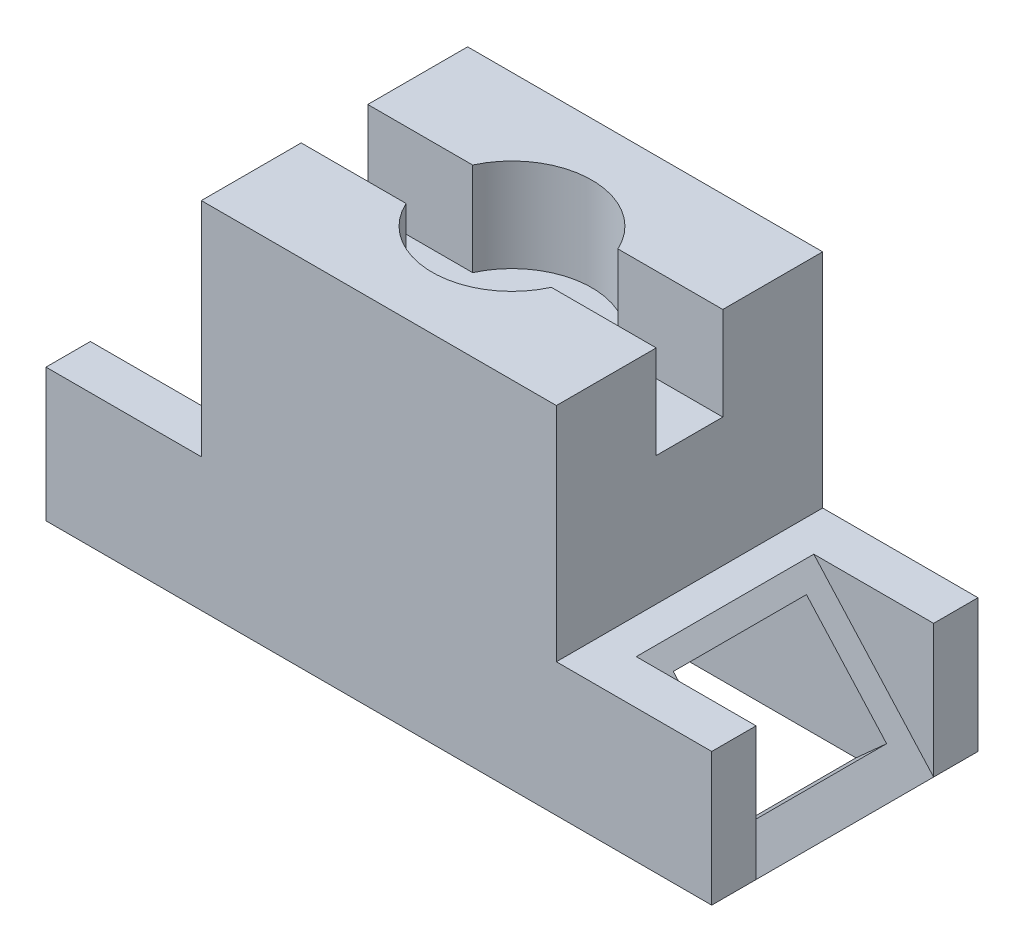
ISO-10303-21;
HEADER;
FILE_DESCRIPTION(('STEP AP214'),'2;1');
FILE_NAME('part.step','',(''),(''),'','','');
FILE_SCHEMA(('AUTOMOTIVE_DESIGN { 1 0 10303 214 1 1 1 1 }'));
ENDSEC;
DATA;
#1=APPLICATION_CONTEXT('core data for automotive mechanical design processes');
#2=APPLICATION_PROTOCOL_DEFINITION('international standard','automotive_design',2000,#1);
#3=PRODUCT_CONTEXT('',#1,'mechanical');
#4=PRODUCT('Part','Part','',(#3));
#5=PRODUCT_RELATED_PRODUCT_CATEGORY('part','',(#4));
#6=PRODUCT_DEFINITION_FORMATION('','',#4);
#7=PRODUCT_DEFINITION_CONTEXT('part definition',#1,'design');
#8=PRODUCT_DEFINITION('design','',#6,#7);
#9=PRODUCT_DEFINITION_SHAPE('','',#8);
#10=(LENGTH_UNIT() NAMED_UNIT(*) SI_UNIT(.MILLI.,.METRE.));
#11=(NAMED_UNIT(*) PLANE_ANGLE_UNIT() SI_UNIT($,.RADIAN.));
#12=(NAMED_UNIT(*) SI_UNIT($,.STERADIAN.) SOLID_ANGLE_UNIT());
#13=UNCERTAINTY_MEASURE_WITH_UNIT(LENGTH_MEASURE(1.E-05),#10,'distance_accuracy_value','');
#14=(GEOMETRIC_REPRESENTATION_CONTEXT(3) GLOBAL_UNCERTAINTY_ASSIGNED_CONTEXT((#13)) GLOBAL_UNIT_ASSIGNED_CONTEXT((#10,
#11,#12)) REPRESENTATION_CONTEXT('',''));
#15=CARTESIAN_POINT('',(0.,0.,0.));
#16=DIRECTION('',(0.,0.,1.));
#17=DIRECTION('',(1.,0.,0.));
#18=AXIS2_PLACEMENT_3D('',#15,#16,#17);
#19=CARTESIAN_POINT('',(-47.8178368121442,-10.,-9.99999999999999));
#20=DIRECTION('',(0.,0.,1.));
#21=DIRECTION('',(1.,0.,0.));
#22=AXIS2_PLACEMENT_3D('',#19,#20,#21);
#23=PLANE('',#22);
#24=DIRECTION('',(-0.707106781186548,-0.707106781186547,0.));
#25=VECTOR('',#24,1.);
#26=CARTESIAN_POINT('',(-47.8178368121442,0.,-10.));
#27=LINE('',#26,#25);
#28=CARTESIAN_POINT('',(-17.8178368121442,30.,-10.));
#29=VERTEX_POINT('',#28);
#30=CARTESIAN_POINT('',(-47.8178368121442,0.,-9.99999999999999));
#31=VERTEX_POINT('',#30);
#32=EDGE_CURVE('E274',#29,#31,#27,.T.);
#33=ORIENTED_EDGE('',*,*,#32,.T.);
#34=DIRECTION('',(0.,1.,0.));
#35=VECTOR('',#34,1.);
#36=CARTESIAN_POINT('',(-47.8178368121442,-10.,-9.99999999999999));
#37=LINE('',#36,#35);
#38=CARTESIAN_POINT('',(-47.8178368121442,30.,-9.99999999999999));
#39=VERTEX_POINT('',#38);
#40=EDGE_CURVE('E289',#31,#39,#37,.T.);
#41=ORIENTED_EDGE('',*,*,#40,.T.);
#42=DIRECTION('',(1.,0.,0.));
#43=VECTOR('',#42,1.);
#44=CARTESIAN_POINT('',(-47.8178368121442,30.,-9.99999999999999));
#45=LINE('',#44,#43);
#46=EDGE_CURVE('E288',#39,#29,#45,.T.);
#47=ORIENTED_EDGE('',*,*,#46,.T.);
#48=EDGE_LOOP('',(#33,#41,#47));
#49=FACE_BOUND('',#48,.T.);
#50=ADVANCED_FACE('F39',(#49),#23,.F.);
#51=CARTESIAN_POINT('',(-47.8178368121442,-10.,-50.));
#52=DIRECTION('',(0.,0.,-1.));
#53=DIRECTION('',(-1.,0.,0.));
#54=AXIS2_PLACEMENT_3D('',#51,#52,#53);
#55=PLANE('',#54);
#56=DIRECTION('',(-0.707106781186548,-0.707106781186547,0.));
#57=VECTOR('',#56,1.);
#58=CARTESIAN_POINT('',(-47.8178368121442,0.,-50.));
#59=LINE('',#58,#57);
#60=CARTESIAN_POINT('',(-17.8178368121442,30.,-50.));
#61=VERTEX_POINT('',#60);
#62=CARTESIAN_POINT('',(-47.8178368121442,0.,-50.));
#63=VERTEX_POINT('',#62);
#64=EDGE_CURVE('E271',#61,#63,#59,.T.);
#65=ORIENTED_EDGE('',*,*,#64,.F.);
#66=DIRECTION('',(-1.,0.,0.));
#67=VECTOR('',#66,1.);
#68=CARTESIAN_POINT('',(-47.8178368121442,30.,-50.));
#69=LINE('',#68,#67);
#70=CARTESIAN_POINT('',(-47.8178368121442,30.,-50.));
#71=VERTEX_POINT('',#70);
#72=EDGE_CURVE('E281',#61,#71,#69,.T.);
#73=ORIENTED_EDGE('',*,*,#72,.T.);
#74=DIRECTION('',(0.,1.,0.));
#75=VECTOR('',#74,1.);
#76=CARTESIAN_POINT('',(-47.8178368121442,-10.,-50.));
#77=LINE('',#76,#75);
#78=EDGE_CURVE('E286',#63,#71,#77,.T.);
#79=ORIENTED_EDGE('',*,*,#78,.F.);
#80=EDGE_LOOP('',(#65,#73,#79));
#81=FACE_BOUND('',#80,.T.);
#82=ADVANCED_FACE('F548',(#81),#55,.F.);
#83=CARTESIAN_POINT('',(-47.8178368121442,30.,-60.));
#84=DIRECTION('',(-1.,0.,0.));
#85=DIRECTION('',(0.,-1.,0.));
#86=AXIS2_PLACEMENT_3D('',#83,#84,#85);
#87=PLANE('',#86);
#88=ORIENTED_EDGE('',*,*,#40,.F.);
#89=DIRECTION('',(0.,0.,1.));
#90=VECTOR('',#89,1.);
#91=CARTESIAN_POINT('',(-47.8178368121442,0.,-60.));
#92=LINE('',#91,#90);
#93=CARTESIAN_POINT('',(-47.8178368121442,0.,0.));
#94=VERTEX_POINT('',#93);
#95=EDGE_CURVE('E420',#31,#94,#92,.T.);
#96=ORIENTED_EDGE('',*,*,#95,.T.);
#97=DIRECTION('',(0.,-1.,0.));
#98=VECTOR('',#97,1.);
#99=CARTESIAN_POINT('',(-47.8178368121442,30.,0.));
#100=LINE('',#99,#98);
#101=CARTESIAN_POINT('',(-47.8178368121442,30.,0.));
#102=VERTEX_POINT('',#101);
#103=EDGE_CURVE('E386',#102,#94,#100,.T.);
#104=ORIENTED_EDGE('',*,*,#103,.F.);
#105=DIRECTION('',(0.,0.,1.));
#106=VECTOR('',#105,1.);
#107=CARTESIAN_POINT('',(-47.8178368121442,30.,-60.));
#108=LINE('',#107,#106);
#109=EDGE_CURVE('E48',#39,#102,#108,.T.);
#110=ORIENTED_EDGE('',*,*,#109,.F.);
#111=EDGE_LOOP('',(#88,#96,#104,#110));
#112=FACE_BOUND('',#111,.T.);
#113=ADVANCED_FACE('F469',(#112),#87,.T.);
#114=CARTESIAN_POINT('',(75.1821631878558,-10.,-50.));
#115=DIRECTION('',(0.,0.,-1.));
#116=DIRECTION('',(-1.,0.,0.));
#117=AXIS2_PLACEMENT_3D('',#114,#115,#116);
#118=PLANE('',#117);
#119=DIRECTION('',(-0.66896473162245,0.743294146247166,0.));
#120=VECTOR('',#119,1.);
#121=CARTESIAN_POINT('',(75.1821631878558,30.,-50.));
#122=LINE('',#121,#120);
#123=CARTESIAN_POINT('',(102.182163187856,0.,-50.));
#124=VERTEX_POINT('',#123);
#125=CARTESIAN_POINT('',(75.1821631878558,30.,-50.));
#126=VERTEX_POINT('',#125);
#127=EDGE_CURVE('E321',#124,#126,#122,.T.);
#128=ORIENTED_EDGE('',*,*,#127,.F.);
#129=DIRECTION('',(0.,1.,0.));
#130=VECTOR('',#129,1.);
#131=CARTESIAN_POINT('',(102.182163187856,-10.,-50.));
#132=LINE('',#131,#130);
#133=CARTESIAN_POINT('',(102.182163187856,30.,-50.));
#134=VERTEX_POINT('',#133);
#135=EDGE_CURVE('E339',#124,#134,#132,.T.);
#136=ORIENTED_EDGE('',*,*,#135,.T.);
#137=DIRECTION('',(-1.,0.,0.));
#138=VECTOR('',#137,1.);
#139=CARTESIAN_POINT('',(75.1821631878558,30.,-50.));
#140=LINE('',#139,#138);
#141=EDGE_CURVE('E333',#134,#126,#140,.T.);
#142=ORIENTED_EDGE('',*,*,#141,.T.);
#143=EDGE_LOOP('',(#128,#136,#142));
#144=FACE_BOUND('',#143,.T.);
#145=ADVANCED_FACE('F513',(#144),#118,.F.);
#146=CARTESIAN_POINT('',(102.182163187856,-10.,-10.));
#147=DIRECTION('',(0.,0.,1.));
#148=DIRECTION('',(1.,0.,0.));
#149=AXIS2_PLACEMENT_3D('',#146,#147,#148);
#150=PLANE('',#149);
#151=DIRECTION('',(-0.66896473162245,0.743294146247166,0.));
#152=VECTOR('',#151,1.);
#153=CARTESIAN_POINT('',(75.1821631878558,30.,-10.));
#154=LINE('',#153,#152);
#155=CARTESIAN_POINT('',(102.182163187856,0.,-10.));
#156=VERTEX_POINT('',#155);
#157=CARTESIAN_POINT('',(75.1821631878558,30.,-10.));
#158=VERTEX_POINT('',#157);
#159=EDGE_CURVE('E325',#156,#158,#154,.T.);
#160=ORIENTED_EDGE('',*,*,#159,.T.);
#161=DIRECTION('',(1.,0.,0.));
#162=VECTOR('',#161,1.);
#163=CARTESIAN_POINT('',(102.182163187856,30.,-10.));
#164=LINE('',#163,#162);
#165=CARTESIAN_POINT('',(102.182163187856,30.,-10.));
#166=VERTEX_POINT('',#165);
#167=EDGE_CURVE('E337',#158,#166,#164,.T.);
#168=ORIENTED_EDGE('',*,*,#167,.T.);
#169=DIRECTION('',(0.,1.,0.));
#170=VECTOR('',#169,1.);
#171=CARTESIAN_POINT('',(102.182163187856,-10.,-10.));
#172=LINE('',#171,#170);
#173=EDGE_CURVE('E336',#156,#166,#172,.T.);
#174=ORIENTED_EDGE('',*,*,#173,.F.);
#175=EDGE_LOOP('',(#160,#168,#174));
#176=FACE_BOUND('',#175,.T.);
#177=ADVANCED_FACE('F517',(#176),#150,.F.);
#178=CARTESIAN_POINT('',(102.182163187856,0.,-60.));
#179=DIRECTION('',(1.,0.,0.));
#180=DIRECTION('',(0.,0.,-1.));
#181=AXIS2_PLACEMENT_3D('',#178,#179,#180);
#182=PLANE('',#181);
#183=ORIENTED_EDGE('',*,*,#135,.F.);
#184=DIRECTION('',(0.,0.,1.));
#185=VECTOR('',#184,1.);
#186=CARTESIAN_POINT('',(102.182163187856,0.,-60.));
#187=LINE('',#186,#185);
#188=CARTESIAN_POINT('',(102.182163187856,0.,-60.));
#189=VERTEX_POINT('',#188);
#190=EDGE_CURVE('E452',#189,#124,#187,.T.);
#191=ORIENTED_EDGE('',*,*,#190,.F.);
#192=DIRECTION('',(0.,1.,0.));
#193=VECTOR('',#192,1.);
#194=CARTESIAN_POINT('',(102.182163187856,0.,-60.));
#195=LINE('',#194,#193);
#196=CARTESIAN_POINT('',(102.182163187856,30.,-60.));
#197=VERTEX_POINT('',#196);
#198=EDGE_CURVE('E399',#189,#197,#195,.T.);
#199=ORIENTED_EDGE('',*,*,#198,.T.);
#200=DIRECTION('',(0.,0.,1.));
#201=VECTOR('',#200,1.);
#202=CARTESIAN_POINT('',(102.182163187856,30.,-60.));
#203=LINE('',#202,#201);
#204=EDGE_CURVE('E451',#197,#134,#203,.T.);
#205=ORIENTED_EDGE('',*,*,#204,.T.);
#206=EDGE_LOOP('',(#183,#191,#199,#205));
#207=FACE_BOUND('',#206,.T.);
#208=ADVANCED_FACE('F514',(#207),#182,.T.);
#209=CARTESIAN_POINT('',(67.1821631878558,80.,-60.));
#210=DIRECTION('',(0.,1.,0.));
#211=DIRECTION('',(-1.,0.,0.));
#212=AXIS2_PLACEMENT_3D('',#209,#210,#211);
#213=PLANE('',#212);
#214=DIRECTION('',(1.,0.,0.));
#215=VECTOR('',#214,1.);
#216=CARTESIAN_POINT('',(-12.8178368121442,80.,-22.5));
#217=LINE('',#216,#215);
#218=CARTESIAN_POINT('',(-12.8178368121442,80.,-22.5));
#219=VERTEX_POINT('',#218);
#220=CARTESIAN_POINT('',(10.8190950159022,80.,-22.5));
#221=VERTEX_POINT('',#220);
#222=EDGE_CURVE('E357',#219,#221,#217,.T.);
#223=ORIENTED_EDGE('',*,*,#222,.F.);
#224=DIRECTION('',(0.,0.,1.));
#225=VECTOR('',#224,1.);
#226=CARTESIAN_POINT('',(-12.8178368121442,80.,-60.));
#227=LINE('',#226,#225);
#228=CARTESIAN_POINT('',(-12.8178368121442,80.,0.));
#229=VERTEX_POINT('',#228);
#230=EDGE_CURVE('E444',#219,#229,#227,.T.);
#231=ORIENTED_EDGE('',*,*,#230,.T.);
#232=DIRECTION('',(-1.,0.,0.));
#233=VECTOR('',#232,1.);
#234=CARTESIAN_POINT('',(67.1821631878558,80.,0.));
#235=LINE('',#234,#233);
#236=CARTESIAN_POINT('',(67.1821631878558,80.,0.));
#237=VERTEX_POINT('',#236);
#238=EDGE_CURVE('E435',#237,#229,#235,.T.);
#239=ORIENTED_EDGE('',*,*,#238,.F.);
#240=DIRECTION('',(0.,0.,1.));
#241=VECTOR('',#240,1.);
#242=CARTESIAN_POINT('',(67.1821631878558,80.,-60.));
#243=LINE('',#242,#241);
#244=CARTESIAN_POINT('',(67.1821631878558,80.,-22.5));
#245=VERTEX_POINT('',#244);
#246=EDGE_CURVE('E446',#245,#237,#243,.T.);
#247=ORIENTED_EDGE('',*,*,#246,.F.);
#248=CARTESIAN_POINT('',(43.5452313598093,80.,-22.5));
#249=VERTEX_POINT('',#248);
#250=EDGE_CURVE('E344',#249,#245,#217,.T.);
#251=ORIENTED_EDGE('',*,*,#250,.F.);
#252=CARTESIAN_POINT('',(27.1821631878558,80.,-30.));
#253=DIRECTION('',(0.,1.,0.));
#254=DIRECTION('',(-1.,0.,0.));
#255=AXIS2_PLACEMENT_3D('',#252,#253,#254);
#256=CIRCLE('',#255,18.);
#257=EDGE_CURVE('E388',#221,#249,#256,.T.);
#258=ORIENTED_EDGE('',*,*,#257,.F.);
#259=EDGE_LOOP('',(#223,#231,#239,#247,#251,#258));
#260=FACE_BOUND('',#259,.T.);
#261=ADVANCED_FACE('F527',(#260),#213,.T.);
#262=CARTESIAN_POINT('',(27.1821631878558,59.,-30.));
#263=DIRECTION('',(0.,1.,0.));
#264=DIRECTION('',(-1.,0.,0.));
#265=AXIS2_PLACEMENT_3D('',#262,#263,#264);
#266=CYLINDRICAL_SURFACE('',#265,18.);
#267=ORIENTED_EDGE('',*,*,#257,.T.);
#268=DIRECTION('',(0.,1.,0.));
#269=VECTOR('',#268,1.);
#270=CARTESIAN_POINT('',(43.5452313598093,59.,-22.5));
#271=LINE('',#270,#269);
#272=CARTESIAN_POINT('',(43.5452313598093,59.,-22.5));
#273=VERTEX_POINT('',#272);
#274=EDGE_CURVE('E379',#249,#273,#271,.F.);
#275=ORIENTED_EDGE('',*,*,#274,.T.);
#276=CARTESIAN_POINT('',(27.1821631878558,59.,-30.));
#277=DIRECTION('',(0.,1.,0.));
#278=DIRECTION('',(-1.,0.,0.));
#279=AXIS2_PLACEMENT_3D('',#276,#277,#278);
#280=CIRCLE('',#279,18.);
#281=CARTESIAN_POINT('',(10.8190950159022,59.,-22.5));
#282=VERTEX_POINT('',#281);
#283=EDGE_CURVE('E381',#282,#273,#280,.T.);
#284=ORIENTED_EDGE('',*,*,#283,.F.);
#285=DIRECTION('',(0.,1.,0.));
#286=VECTOR('',#285,1.);
#287=CARTESIAN_POINT('',(10.8190950159022,59.,-22.5));
#288=LINE('',#287,#286);
#289=EDGE_CURVE('E380',#282,#221,#288,.T.);
#290=ORIENTED_EDGE('',*,*,#289,.T.);
#291=EDGE_LOOP('',(#267,#275,#284,#290));
#292=FACE_BOUND('',#291,.T.);
#293=ADVANCED_FACE('F596',(#292),#266,.F.);
#294=ORIENTED_EDGE('',*,*,#78,.T.);
#295=CARTESIAN_POINT('',(-47.8178368121442,30.,-60.));
#296=VERTEX_POINT('',#295);
#297=EDGE_CURVE('E11',#296,#71,#108,.T.);
#298=ORIENTED_EDGE('',*,*,#297,.F.);
#299=DIRECTION('',(0.,-1.,0.));
#300=VECTOR('',#299,1.);
#301=CARTESIAN_POINT('',(-47.8178368121442,30.,-60.));
#302=LINE('',#301,#300);
#303=CARTESIAN_POINT('',(-47.8178368121442,0.,-60.));
#304=VERTEX_POINT('',#303);
#305=EDGE_CURVE('E395',#296,#304,#302,.T.);
#306=ORIENTED_EDGE('',*,*,#305,.T.);
#307=EDGE_CURVE('E43',#304,#63,#92,.T.);
#308=ORIENTED_EDGE('',*,*,#307,.T.);
#309=EDGE_LOOP('',(#294,#298,#306,#308));
#310=FACE_BOUND('',#309,.T.);
#311=ADVANCED_FACE('F41',(#310),#87,.T.);
#312=CARTESIAN_POINT('',(-12.8178368121442,30.,-60.));
#313=DIRECTION('',(0.,1.,0.));
#314=DIRECTION('',(0.,0.,1.));
#315=AXIS2_PLACEMENT_3D('',#312,#313,#314);
#316=PLANE('',#315);
#317=ORIENTED_EDGE('',*,*,#46,.F.);
#318=ORIENTED_EDGE('',*,*,#109,.T.);
#319=DIRECTION('',(-1.,0.,0.));
#320=VECTOR('',#319,1.);
#321=CARTESIAN_POINT('',(-12.8178368121442,30.,0.));
#322=LINE('',#321,#320);
#323=CARTESIAN_POINT('',(-12.8178368121442,30.,0.));
#324=VERTEX_POINT('',#323);
#325=EDGE_CURVE('E398',#324,#102,#322,.T.);
#326=ORIENTED_EDGE('',*,*,#325,.F.);
#327=DIRECTION('',(0.,0.,1.));
#328=VECTOR('',#327,1.);
#329=CARTESIAN_POINT('',(-12.8178368121442,30.,-60.));
#330=LINE('',#329,#328);
#331=CARTESIAN_POINT('',(-12.8178368121442,30.,-60.));
#332=VERTEX_POINT('',#331);
#333=EDGE_CURVE('E439',#332,#324,#330,.T.);
#334=ORIENTED_EDGE('',*,*,#333,.F.);
#335=DIRECTION('',(-1.,0.,0.));
#336=VECTOR('',#335,1.);
#337=CARTESIAN_POINT('',(-12.8178368121442,30.,-60.));
#338=LINE('',#337,#336);
#339=EDGE_CURVE('E411',#332,#296,#338,.T.);
#340=ORIENTED_EDGE('',*,*,#339,.T.);
#341=ORIENTED_EDGE('',*,*,#297,.T.);
#342=ORIENTED_EDGE('',*,*,#72,.F.);
#343=DIRECTION('',(0.,0.,-1.));
#344=VECTOR('',#343,1.);
#345=CARTESIAN_POINT('',(-17.8178368121442,30.,-50.));
#346=LINE('',#345,#344);
#347=EDGE_CURVE('E282',#29,#61,#346,.T.);
#348=ORIENTED_EDGE('',*,*,#347,.F.);
#349=EDGE_LOOP('',(#317,#318,#326,#334,#340,#341,#342,#348));
#350=FACE_BOUND('',#349,.T.);
#351=ADVANCED_FACE('F478',(#350),#316,.T.);
#352=CARTESIAN_POINT('',(-12.8178368121442,80.,-60.));
#353=DIRECTION('',(-1.,0.,0.));
#354=DIRECTION('',(0.,-1.,0.));
#355=AXIS2_PLACEMENT_3D('',#352,#353,#354);
#356=PLANE('',#355);
#357=DIRECTION('',(0.,1.,0.));
#358=VECTOR('',#357,1.);
#359=CARTESIAN_POINT('',(-12.8178368121442,59.,-22.5));
#360=LINE('',#359,#358);
#361=CARTESIAN_POINT('',(-12.8178368121442,59.,-22.5));
#362=VERTEX_POINT('',#361);
#363=EDGE_CURVE('E365',#362,#219,#360,.T.);
#364=ORIENTED_EDGE('',*,*,#363,.F.);
#365=DIRECTION('',(0.,0.,1.));
#366=VECTOR('',#365,1.);
#367=CARTESIAN_POINT('',(-12.8178368121442,59.,-37.5));
#368=LINE('',#367,#366);
#369=CARTESIAN_POINT('',(-12.8178368121442,59.,-37.5));
#370=VERTEX_POINT('',#369);
#371=EDGE_CURVE('E351',#370,#362,#368,.T.);
#372=ORIENTED_EDGE('',*,*,#371,.F.);
#373=DIRECTION('',(0.,1.,0.));
#374=VECTOR('',#373,1.);
#375=CARTESIAN_POINT('',(-12.8178368121442,59.,-37.5));
#376=LINE('',#375,#374);
#377=CARTESIAN_POINT('',(-12.8178368121442,80.,-37.5));
#378=VERTEX_POINT('',#377);
#379=EDGE_CURVE('E362',#370,#378,#376,.T.);
#380=ORIENTED_EDGE('',*,*,#379,.T.);
#381=CARTESIAN_POINT('',(-12.8178368121442,80.,-60.));
#382=VERTEX_POINT('',#381);
#383=EDGE_CURVE('E445',#382,#378,#227,.T.);
#384=ORIENTED_EDGE('',*,*,#383,.F.);
#385=DIRECTION('',(0.,-1.,0.));
#386=VECTOR('',#385,1.);
#387=CARTESIAN_POINT('',(-12.8178368121442,80.,-60.));
#388=LINE('',#387,#386);
#389=EDGE_CURVE('E412',#382,#332,#388,.T.);
#390=ORIENTED_EDGE('',*,*,#389,.T.);
#391=ORIENTED_EDGE('',*,*,#333,.T.);
#392=DIRECTION('',(0.,-1.,0.));
#393=VECTOR('',#392,1.);
#394=CARTESIAN_POINT('',(-12.8178368121442,80.,0.));
#395=LINE('',#394,#393);
#396=EDGE_CURVE('E434',#229,#324,#395,.T.);
#397=ORIENTED_EDGE('',*,*,#396,.F.);
#398=ORIENTED_EDGE('',*,*,#230,.F.);
#399=EDGE_LOOP('',(#364,#372,#380,#384,#390,#391,#397,#398));
#400=FACE_BOUND('',#399,.T.);
#401=ADVANCED_FACE('F534',(#400),#356,.T.);
#402=DIRECTION('',(-1.,0.,0.));
#403=VECTOR('',#402,1.);
#404=CARTESIAN_POINT('',(-12.8178368121442,80.,-37.5));
#405=LINE('',#404,#403);
#406=CARTESIAN_POINT('',(67.1821631878558,80.,-37.5));
#407=VERTEX_POINT('',#406);
#408=CARTESIAN_POINT('',(43.5452313598093,80.,-37.5));
#409=VERTEX_POINT('',#408);
#410=EDGE_CURVE('E359',#407,#409,#405,.T.);
#411=ORIENTED_EDGE('',*,*,#410,.F.);
#412=CARTESIAN_POINT('',(67.1821631878558,80.,-60.));
#413=VERTEX_POINT('',#412);
#414=EDGE_CURVE('E447',#413,#407,#243,.T.);
#415=ORIENTED_EDGE('',*,*,#414,.F.);
#416=DIRECTION('',(-1.,0.,0.));
#417=VECTOR('',#416,1.);
#418=CARTESIAN_POINT('',(67.1821631878558,80.,-60.));
#419=LINE('',#418,#417);
#420=EDGE_CURVE('E410',#413,#382,#419,.T.);
#421=ORIENTED_EDGE('',*,*,#420,.T.);
#422=ORIENTED_EDGE('',*,*,#383,.T.);
#423=CARTESIAN_POINT('',(10.8190950159022,80.,-37.5));
#424=VERTEX_POINT('',#423);
#425=EDGE_CURVE('E360',#424,#378,#405,.T.);
#426=ORIENTED_EDGE('',*,*,#425,.F.);
#427=EDGE_CURVE('E384',#409,#424,#256,.T.);
#428=ORIENTED_EDGE('',*,*,#427,.F.);
#429=EDGE_LOOP('',(#411,#415,#421,#422,#426,#428));
#430=FACE_BOUND('',#429,.T.);
#431=ADVANCED_FACE('F498',(#430),#213,.T.);
#432=CARTESIAN_POINT('',(67.1821631878558,30.,-60.));
#433=DIRECTION('',(1.,0.,0.));
#434=DIRECTION('',(0.,0.,-1.));
#435=AXIS2_PLACEMENT_3D('',#432,#433,#434);
#436=PLANE('',#435);
#437=DIRECTION('',(0.,1.,0.));
#438=VECTOR('',#437,1.);
#439=CARTESIAN_POINT('',(67.1821631878558,59.,-22.5));
#440=LINE('',#439,#438);
#441=CARTESIAN_POINT('',(67.1821631878558,59.,-22.5));
#442=VERTEX_POINT('',#441);
#443=EDGE_CURVE('E358',#442,#245,#440,.T.);
#444=ORIENTED_EDGE('',*,*,#443,.T.);
#445=ORIENTED_EDGE('',*,*,#246,.T.);
#446=DIRECTION('',(0.,1.,0.));
#447=VECTOR('',#446,1.);
#448=CARTESIAN_POINT('',(67.1821631878558,30.,0.));
#449=LINE('',#448,#447);
#450=CARTESIAN_POINT('',(67.1821631878558,30.,0.));
#451=VERTEX_POINT('',#450);
#452=EDGE_CURVE('E429',#451,#237,#449,.T.);
#453=ORIENTED_EDGE('',*,*,#452,.F.);
#454=DIRECTION('',(0.,0.,1.));
#455=VECTOR('',#454,1.);
#456=CARTESIAN_POINT('',(67.1821631878558,30.,-60.));
#457=LINE('',#456,#455);
#458=CARTESIAN_POINT('',(67.1821631878558,30.,-60.));
#459=VERTEX_POINT('',#458);
#460=EDGE_CURVE('E448',#459,#451,#457,.T.);
#461=ORIENTED_EDGE('',*,*,#460,.F.);
#462=DIRECTION('',(0.,1.,0.));
#463=VECTOR('',#462,1.);
#464=CARTESIAN_POINT('',(67.1821631878558,30.,-60.));
#465=LINE('',#464,#463);
#466=EDGE_CURVE('E403',#459,#413,#465,.T.);
#467=ORIENTED_EDGE('',*,*,#466,.T.);
#468=ORIENTED_EDGE('',*,*,#414,.T.);
#469=DIRECTION('',(0.,1.,0.));
#470=VECTOR('',#469,1.);
#471=CARTESIAN_POINT('',(67.1821631878558,59.,-37.5));
#472=LINE('',#471,#470);
#473=CARTESIAN_POINT('',(67.1821631878558,59.,-37.5));
#474=VERTEX_POINT('',#473);
#475=EDGE_CURVE('E368',#474,#407,#472,.T.);
#476=ORIENTED_EDGE('',*,*,#475,.F.);
#477=DIRECTION('',(0.,0.,-1.));
#478=VECTOR('',#477,1.);
#479=CARTESIAN_POINT('',(67.1821631878558,59.,-37.5));
#480=LINE('',#479,#478);
#481=EDGE_CURVE('E347',#442,#474,#480,.T.);
#482=ORIENTED_EDGE('',*,*,#481,.F.);
#483=EDGE_LOOP('',(#444,#445,#453,#461,#467,#468,#476,#482));
#484=FACE_BOUND('',#483,.T.);
#485=ADVANCED_FACE('F503',(#484),#436,.T.);
#486=CARTESIAN_POINT('',(102.182163187856,30.,-60.));
#487=DIRECTION('',(0.,1.,0.));
#488=DIRECTION('',(-1.,0.,0.));
#489=AXIS2_PLACEMENT_3D('',#486,#487,#488);
#490=PLANE('',#489);
#491=ORIENTED_EDGE('',*,*,#141,.F.);
#492=ORIENTED_EDGE('',*,*,#204,.F.);
#493=DIRECTION('',(-1.,0.,0.));
#494=VECTOR('',#493,1.);
#495=CARTESIAN_POINT('',(102.182163187856,30.,-60.));
#496=LINE('',#495,#494);
#497=EDGE_CURVE('E405',#197,#459,#496,.T.);
#498=ORIENTED_EDGE('',*,*,#497,.T.);
#499=ORIENTED_EDGE('',*,*,#460,.T.);
#500=DIRECTION('',(-1.,0.,0.));
#501=VECTOR('',#500,1.);
#502=CARTESIAN_POINT('',(102.182163187856,30.,0.));
#503=LINE('',#502,#501);
#504=CARTESIAN_POINT('',(102.182163187856,30.,0.));
#505=VERTEX_POINT('',#504);
#506=EDGE_CURVE('E428',#505,#451,#503,.T.);
#507=ORIENTED_EDGE('',*,*,#506,.F.);
#508=EDGE_CURVE('E453',#166,#505,#203,.T.);
#509=ORIENTED_EDGE('',*,*,#508,.F.);
#510=ORIENTED_EDGE('',*,*,#167,.F.);
#511=DIRECTION('',(0.,0.,1.));
#512=VECTOR('',#511,1.);
#513=CARTESIAN_POINT('',(75.1821631878558,30.,-10.));
#514=LINE('',#513,#512);
#515=EDGE_CURVE('E331',#126,#158,#514,.T.);
#516=ORIENTED_EDGE('',*,*,#515,.F.);
#517=EDGE_LOOP('',(#491,#492,#498,#499,#507,#509,#510,#516));
#518=FACE_BOUND('',#517,.T.);
#519=ADVANCED_FACE('F507',(#518),#490,.T.);
#520=ORIENTED_EDGE('',*,*,#173,.T.);
#521=ORIENTED_EDGE('',*,*,#508,.T.);
#522=DIRECTION('',(0.,1.,0.));
#523=VECTOR('',#522,1.);
#524=CARTESIAN_POINT('',(102.182163187856,0.,0.));
#525=LINE('',#524,#523);
#526=CARTESIAN_POINT('',(102.182163187856,0.,0.));
#527=VERTEX_POINT('',#526);
#528=EDGE_CURVE('E421',#527,#505,#525,.T.);
#529=ORIENTED_EDGE('',*,*,#528,.F.);
#530=EDGE_CURVE('E460',#156,#527,#187,.T.);
#531=ORIENTED_EDGE('',*,*,#530,.F.);
#532=EDGE_LOOP('',(#520,#521,#529,#531));
#533=FACE_BOUND('',#532,.T.);
#534=ADVANCED_FACE('F524',(#533),#182,.T.);
#535=CARTESIAN_POINT('',(-47.8178368121442,0.,-60.));
#536=DIRECTION('',(0.,-1.,0.));
#537=DIRECTION('',(0.,0.,-1.));
#538=AXIS2_PLACEMENT_3D('',#535,#536,#537);
#539=PLANE('',#538);
#540=DIRECTION('',(-1.,0.,0.));
#541=VECTOR('',#540,1.);
#542=CARTESIAN_POINT('',(-47.8178368121442,0.,-15.));
#543=LINE('',#542,#541);
#544=CARTESIAN_POINT('',(5.11109537599028,0.,-15.));
#545=VERTEX_POINT('',#544);
#546=CARTESIAN_POINT('',(-33.0726708080833,0.,-15.));
#547=VERTEX_POINT('',#546);
#548=EDGE_CURVE('E272',#545,#547,#543,.T.);
#549=ORIENTED_EDGE('',*,*,#548,.F.);
#550=DIRECTION('',(0.,0.,1.));
#551=VECTOR('',#550,1.);
#552=CARTESIAN_POINT('',(5.11109537599028,0.,-60.));
#553=LINE('',#552,#551);
#554=CARTESIAN_POINT('',(5.11109537599028,0.,-45.));
#555=VERTEX_POINT('',#554);
#556=EDGE_CURVE('E261',#555,#545,#553,.T.);
#557=ORIENTED_EDGE('',*,*,#556,.F.);
#558=DIRECTION('',(1.,0.,0.));
#559=VECTOR('',#558,1.);
#560=CARTESIAN_POINT('',(-47.8178368121442,0.,-45.));
#561=LINE('',#560,#559);
#562=CARTESIAN_POINT('',(-33.0726708080833,0.,-45.));
#563=VERTEX_POINT('',#562);
#564=EDGE_CURVE('E242',#563,#555,#561,.T.);
#565=ORIENTED_EDGE('',*,*,#564,.F.);
#566=DIRECTION('',(0.,0.,-1.));
#567=VECTOR('',#566,1.);
#568=CARTESIAN_POINT('',(-33.0726708080833,0.,-60.));
#569=LINE('',#568,#567);
#570=EDGE_CURVE('E269',#547,#563,#569,.T.);
#571=ORIENTED_EDGE('',*,*,#570,.F.);
#572=EDGE_LOOP('',(#549,#557,#565,#571));
#573=FACE_BOUND('',#572,.T.);
#574=ORIENTED_EDGE('',*,*,#95,.F.);
#575=DIRECTION('',(0.,0.,-1.));
#576=VECTOR('',#575,1.);
#577=CARTESIAN_POINT('',(-47.8178368121442,0.,-10.));
#578=LINE('',#577,#576);
#579=EDGE_CURVE('E279',#31,#63,#578,.T.);
#580=ORIENTED_EDGE('',*,*,#579,.T.);
#581=ORIENTED_EDGE('',*,*,#307,.F.);
#582=DIRECTION('',(1.,0.,0.));
#583=VECTOR('',#582,1.);
#584=CARTESIAN_POINT('',(-47.8178368121442,0.,-60.));
#585=LINE('',#584,#583);
#586=EDGE_CURVE('E393',#304,#189,#585,.T.);
#587=ORIENTED_EDGE('',*,*,#586,.T.);
#588=ORIENTED_EDGE('',*,*,#190,.T.);
#589=DIRECTION('',(0.,0.,-1.));
#590=VECTOR('',#589,1.);
#591=CARTESIAN_POINT('',(102.182163187856,0.,-10.));
#592=LINE('',#591,#590);
#593=EDGE_CURVE('E327',#156,#124,#592,.T.);
#594=ORIENTED_EDGE('',*,*,#593,.F.);
#595=ORIENTED_EDGE('',*,*,#530,.T.);
#596=DIRECTION('',(1.,0.,0.));
#597=VECTOR('',#596,1.);
#598=CARTESIAN_POINT('',(-47.8178368121442,0.,0.));
#599=LINE('',#598,#597);
#600=EDGE_CURVE('E417',#94,#527,#599,.T.);
#601=ORIENTED_EDGE('',*,*,#600,.F.);
#602=EDGE_LOOP('',(#574,#580,#581,#587,#588,#594,#595,#601));
#603=FACE_BOUND('',#602,.T.);
#604=DIRECTION('',(1.,0.,0.));
#605=VECTOR('',#604,1.);
#606=CARTESIAN_POINT('',(-47.8178368121442,0.,-45.));
#607=LINE('',#606,#605);
#608=CARTESIAN_POINT('',(49.3230654362301,0.,-45.));
#609=VERTEX_POINT('',#608);
#610=CARTESIAN_POINT('',(89.6839375774512,0.,-45.));
#611=VERTEX_POINT('',#610);
#612=EDGE_CURVE('E318',#609,#611,#607,.T.);
#613=ORIENTED_EDGE('',*,*,#612,.F.);
#614=DIRECTION('',(0.,0.,-1.));
#615=VECTOR('',#614,1.);
#616=CARTESIAN_POINT('',(49.3230654362301,0.,-60.));
#617=LINE('',#616,#615);
#618=CARTESIAN_POINT('',(49.3230654362301,0.,-15.));
#619=VERTEX_POINT('',#618);
#620=EDGE_CURVE('E310',#619,#609,#617,.T.);
#621=ORIENTED_EDGE('',*,*,#620,.F.);
#622=DIRECTION('',(-1.,0.,0.));
#623=VECTOR('',#622,1.);
#624=CARTESIAN_POINT('',(-47.8178368121442,0.,-15.));
#625=LINE('',#624,#623);
#626=CARTESIAN_POINT('',(89.6839375774512,0.,-15.));
#627=VERTEX_POINT('',#626);
#628=EDGE_CURVE('E314',#627,#619,#625,.T.);
#629=ORIENTED_EDGE('',*,*,#628,.F.);
#630=DIRECTION('',(0.,0.,1.));
#631=VECTOR('',#630,1.);
#632=CARTESIAN_POINT('',(89.6839375774512,0.,-60.));
#633=LINE('',#632,#631);
#634=EDGE_CURVE('E319',#611,#627,#633,.T.);
#635=ORIENTED_EDGE('',*,*,#634,.F.);
#636=EDGE_LOOP('',(#613,#621,#629,#635));
#637=FACE_BOUND('',#636,.T.);
#638=ADVANCED_FACE('F471',(#573,#603,#637),#539,.T.);
#639=CARTESIAN_POINT('',(0.,0.,-60.));
#640=DIRECTION('',(0.,0.,1.));
#641=DIRECTION('',(1.,0.,0.));
#642=AXIS2_PLACEMENT_3D('',#639,#640,#641);
#643=PLANE('',#642);
#644=ORIENTED_EDGE('',*,*,#305,.F.);
#645=ORIENTED_EDGE('',*,*,#339,.F.);
#646=ORIENTED_EDGE('',*,*,#389,.F.);
#647=ORIENTED_EDGE('',*,*,#420,.F.);
#648=ORIENTED_EDGE('',*,*,#466,.F.);
#649=ORIENTED_EDGE('',*,*,#497,.F.);
#650=ORIENTED_EDGE('',*,*,#198,.F.);
#651=ORIENTED_EDGE('',*,*,#586,.F.);
#652=EDGE_LOOP('',(#644,#645,#646,#647,#648,#649,#650,#651));
#653=FACE_BOUND('',#652,.T.);
#654=ADVANCED_FACE('F490',(#653),#643,.F.);
#655=CARTESIAN_POINT('',(0.,0.,0.));
#656=DIRECTION('',(0.,0.,1.));
#657=DIRECTION('',(1.,0.,0.));
#658=AXIS2_PLACEMENT_3D('',#655,#656,#657);
#659=PLANE('',#658);
#660=ORIENTED_EDGE('',*,*,#103,.T.);
#661=ORIENTED_EDGE('',*,*,#600,.T.);
#662=ORIENTED_EDGE('',*,*,#528,.T.);
#663=ORIENTED_EDGE('',*,*,#506,.T.);
#664=ORIENTED_EDGE('',*,*,#452,.T.);
#665=ORIENTED_EDGE('',*,*,#238,.T.);
#666=ORIENTED_EDGE('',*,*,#396,.T.);
#667=ORIENTED_EDGE('',*,*,#325,.T.);
#668=EDGE_LOOP('',(#660,#661,#662,#663,#664,#665,#666,#667));
#669=FACE_BOUND('',#668,.T.);
#670=ADVANCED_FACE('F472',(#669),#659,.T.);
#671=ORIENTED_EDGE('',*,*,#427,.T.);
#672=DIRECTION('',(0.,1.,0.));
#673=VECTOR('',#672,1.);
#674=CARTESIAN_POINT('',(10.8190950159022,59.,-37.5));
#675=LINE('',#674,#673);
#676=CARTESIAN_POINT('',(10.8190950159022,59.,-37.5));
#677=VERTEX_POINT('',#676);
#678=EDGE_CURVE('E372',#424,#677,#675,.F.);
#679=ORIENTED_EDGE('',*,*,#678,.T.);
#680=CARTESIAN_POINT('',(43.5452313598093,59.,-37.5));
#681=VERTEX_POINT('',#680);
#682=EDGE_CURVE('E390',#681,#677,#280,.T.);
#683=ORIENTED_EDGE('',*,*,#682,.F.);
#684=DIRECTION('',(0.,1.,0.));
#685=VECTOR('',#684,1.);
#686=CARTESIAN_POINT('',(43.5452313598093,59.,-37.5));
#687=LINE('',#686,#685);
#688=EDGE_CURVE('E364',#681,#409,#687,.T.);
#689=ORIENTED_EDGE('',*,*,#688,.T.);
#690=EDGE_LOOP('',(#671,#679,#683,#689));
#691=FACE_BOUND('',#690,.T.);
#692=ADVANCED_FACE('F591',(#691),#266,.F.);
#693=CARTESIAN_POINT('',(27.1821631878558,59.,-30.));
#694=DIRECTION('',(0.,1.,0.));
#695=DIRECTION('',(-1.,0.,0.));
#696=AXIS2_PLACEMENT_3D('',#693,#694,#695);
#697=PLANE('',#696);
#698=ORIENTED_EDGE('',*,*,#682,.T.);
#699=DIRECTION('',(-1.,0.,0.));
#700=VECTOR('',#699,1.);
#701=CARTESIAN_POINT('',(-12.8178368121442,59.,-37.5));
#702=LINE('',#701,#700);
#703=EDGE_CURVE('E348',#677,#370,#702,.T.);
#704=ORIENTED_EDGE('',*,*,#703,.T.);
#705=ORIENTED_EDGE('',*,*,#371,.T.);
#706=DIRECTION('',(1.,0.,0.));
#707=VECTOR('',#706,1.);
#708=CARTESIAN_POINT('',(-12.8178368121442,59.,-22.5));
#709=LINE('',#708,#707);
#710=EDGE_CURVE('E343',#362,#282,#709,.T.);
#711=ORIENTED_EDGE('',*,*,#710,.T.);
#712=ORIENTED_EDGE('',*,*,#283,.T.);
#713=EDGE_CURVE('E350',#273,#442,#709,.T.);
#714=ORIENTED_EDGE('',*,*,#713,.T.);
#715=ORIENTED_EDGE('',*,*,#481,.T.);
#716=EDGE_CURVE('E353',#474,#681,#702,.T.);
#717=ORIENTED_EDGE('',*,*,#716,.T.);
#718=EDGE_LOOP('',(#698,#704,#705,#711,#712,#714,#715,#717));
#719=FACE_BOUND('',#718,.T.);
#720=ADVANCED_FACE('F588',(#719),#697,.T.);
#721=CARTESIAN_POINT('',(-12.8178368121442,59.,-37.5));
#722=DIRECTION('',(0.,0.,-1.));
#723=DIRECTION('',(-1.,0.,0.));
#724=AXIS2_PLACEMENT_3D('',#721,#722,#723);
#725=PLANE('',#724);
#726=ORIENTED_EDGE('',*,*,#716,.F.);
#727=ORIENTED_EDGE('',*,*,#475,.T.);
#728=ORIENTED_EDGE('',*,*,#410,.T.);
#729=ORIENTED_EDGE('',*,*,#688,.F.);
#730=EDGE_LOOP('',(#726,#727,#728,#729));
#731=FACE_BOUND('',#730,.T.);
#732=ADVANCED_FACE('F582',(#731),#725,.F.);
#733=CARTESIAN_POINT('',(-12.8178368121442,59.,-22.5));
#734=DIRECTION('',(0.,0.,1.));
#735=DIRECTION('',(1.,0.,0.));
#736=AXIS2_PLACEMENT_3D('',#733,#734,#735);
#737=PLANE('',#736);
#738=ORIENTED_EDGE('',*,*,#250,.T.);
#739=ORIENTED_EDGE('',*,*,#443,.F.);
#740=ORIENTED_EDGE('',*,*,#713,.F.);
#741=ORIENTED_EDGE('',*,*,#274,.F.);
#742=EDGE_LOOP('',(#738,#739,#740,#741));
#743=FACE_BOUND('',#742,.T.);
#744=ADVANCED_FACE('F587',(#743),#737,.F.);
#745=ORIENTED_EDGE('',*,*,#710,.F.);
#746=ORIENTED_EDGE('',*,*,#363,.T.);
#747=ORIENTED_EDGE('',*,*,#222,.T.);
#748=ORIENTED_EDGE('',*,*,#289,.F.);
#749=EDGE_LOOP('',(#745,#746,#747,#748));
#750=FACE_BOUND('',#749,.T.);
#751=ADVANCED_FACE('F585',(#750),#737,.F.);
#752=ORIENTED_EDGE('',*,*,#425,.T.);
#753=ORIENTED_EDGE('',*,*,#379,.F.);
#754=ORIENTED_EDGE('',*,*,#703,.F.);
#755=ORIENTED_EDGE('',*,*,#678,.F.);
#756=EDGE_LOOP('',(#752,#753,#754,#755));
#757=FACE_BOUND('',#756,.T.);
#758=ADVANCED_FACE('F574',(#757),#725,.F.);
#759=CARTESIAN_POINT('',(75.1821631878558,30.,-10.));
#760=DIRECTION('',(-0.743294146247166,-0.66896473162245,0.));
#761=DIRECTION('',(0.66896473162245,-0.743294146247166,0.));
#762=AXIS2_PLACEMENT_3D('',#759,#760,#761);
#763=PLANE('',#762);
#764=DIRECTION('',(0.,0.,1.));
#765=VECTOR('',#764,1.);
#766=CARTESIAN_POINT('',(78.5269868459681,26.2835292687642,-15.));
#767=LINE('',#766,#765);
#768=CARTESIAN_POINT('',(78.526986845968,26.2835292687642,-45.));
#769=VERTEX_POINT('',#768);
#770=CARTESIAN_POINT('',(78.5269868459681,26.2835292687642,-15.));
#771=VERTEX_POINT('',#770);
#772=EDGE_CURVE('E294',#769,#771,#767,.T.);
#773=ORIENTED_EDGE('',*,*,#772,.F.);
#774=DIRECTION('',(-0.66896473162245,0.743294146247166,0.));
#775=VECTOR('',#774,1.);
#776=CARTESIAN_POINT('',(78.5269868459681,26.2835292687642,-45.));
#777=LINE('',#776,#775);
#778=CARTESIAN_POINT('',(96.5890345997742,6.21458732009069,-45.));
#779=VERTEX_POINT('',#778);
#780=EDGE_CURVE('E293',#779,#769,#777,.T.);
#781=ORIENTED_EDGE('',*,*,#780,.F.);
#782=DIRECTION('',(0.,0.,-1.));
#783=VECTOR('',#782,1.);
#784=CARTESIAN_POINT('',(96.5890345997742,6.21458732009069,-15.));
#785=LINE('',#784,#783);
#786=CARTESIAN_POINT('',(96.5890345997742,6.21458732009069,-15.));
#787=VERTEX_POINT('',#786);
#788=EDGE_CURVE('E301',#787,#779,#785,.T.);
#789=ORIENTED_EDGE('',*,*,#788,.F.);
#790=DIRECTION('',(0.66896473162245,-0.743294146247166,0.));
#791=VECTOR('',#790,1.);
#792=CARTESIAN_POINT('',(78.5269868459681,26.2835292687642,-15.));
#793=LINE('',#792,#791);
#794=EDGE_CURVE('E296',#771,#787,#793,.T.);
#795=ORIENTED_EDGE('',*,*,#794,.F.);
#796=EDGE_LOOP('',(#773,#781,#789,#795));
#797=FACE_BOUND('',#796,.T.);
#798=ORIENTED_EDGE('',*,*,#127,.T.);
#799=ORIENTED_EDGE('',*,*,#515,.T.);
#800=ORIENTED_EDGE('',*,*,#159,.F.);
#801=ORIENTED_EDGE('',*,*,#593,.T.);
#802=EDGE_LOOP('',(#798,#799,#800,#801));
#803=FACE_BOUND('',#802,.T.);
#804=ADVANCED_FACE('F516',(#797,#803),#763,.F.);
#805=CARTESIAN_POINT('',(48.7952209960814,-0.475059996133818,-45.));
#806=DIRECTION('',(0.,0.,-1.));
#807=DIRECTION('',(0.,1.,0.));
#808=AXIS2_PLACEMENT_3D('',#805,#806,#807);
#809=PLANE('',#808);
#810=ORIENTED_EDGE('',*,*,#612,.T.);
#811=DIRECTION('',(0.743294146247166,0.66896473162245,0.));
#812=VECTOR('',#811,1.);
#813=CARTESIAN_POINT('',(66.8572687498876,-20.5440019448073,-45.));
#814=LINE('',#813,#812);
#815=EDGE_CURVE('E304',#611,#779,#814,.T.);
#816=ORIENTED_EDGE('',*,*,#815,.T.);
#817=ORIENTED_EDGE('',*,*,#780,.T.);
#818=DIRECTION('',(0.743294146247166,0.66896473162245,0.));
#819=VECTOR('',#818,1.);
#820=CARTESIAN_POINT('',(48.7952209960814,-0.475059996133818,-45.));
#821=LINE('',#820,#819);
#822=EDGE_CURVE('E302',#609,#769,#821,.T.);
#823=ORIENTED_EDGE('',*,*,#822,.F.);
#824=EDGE_LOOP('',(#810,#816,#817,#823));
#825=FACE_BOUND('',#824,.T.);
#826=ADVANCED_FACE('F561',(#825),#809,.F.);
#827=CARTESIAN_POINT('',(66.8572687498876,-20.5440019448073,-15.));
#828=DIRECTION('',(0.66896473162245,-0.743294146247166,0.));
#829=DIRECTION('',(0.743294146247166,0.66896473162245,0.));
#830=AXIS2_PLACEMENT_3D('',#827,#828,#829);
#831=PLANE('',#830);
#832=ORIENTED_EDGE('',*,*,#634,.T.);
#833=DIRECTION('',(0.743294146247166,0.66896473162245,0.));
#834=VECTOR('',#833,1.);
#835=CARTESIAN_POINT('',(66.8572687498876,-20.5440019448073,-15.));
#836=LINE('',#835,#834);
#837=EDGE_CURVE('E308',#627,#787,#836,.T.);
#838=ORIENTED_EDGE('',*,*,#837,.T.);
#839=ORIENTED_EDGE('',*,*,#788,.T.);
#840=ORIENTED_EDGE('',*,*,#815,.F.);
#841=EDGE_LOOP('',(#832,#838,#839,#840));
#842=FACE_BOUND('',#841,.T.);
#843=ADVANCED_FACE('F560',(#842),#831,.F.);
#844=CARTESIAN_POINT('',(48.7952209960814,-0.475059996133818,-15.));
#845=DIRECTION('',(0.,0.,1.));
#846=DIRECTION('',(0.,-1.,0.));
#847=AXIS2_PLACEMENT_3D('',#844,#845,#846);
#848=PLANE('',#847);
#849=ORIENTED_EDGE('',*,*,#628,.T.);
#850=DIRECTION('',(0.743294146247166,0.66896473162245,0.));
#851=VECTOR('',#850,1.);
#852=CARTESIAN_POINT('',(48.7952209960814,-0.475059996133818,-15.));
#853=LINE('',#852,#851);
#854=EDGE_CURVE('E309',#619,#771,#853,.T.);
#855=ORIENTED_EDGE('',*,*,#854,.T.);
#856=ORIENTED_EDGE('',*,*,#794,.T.);
#857=ORIENTED_EDGE('',*,*,#837,.F.);
#858=EDGE_LOOP('',(#849,#855,#856,#857));
#859=FACE_BOUND('',#858,.T.);
#860=ADVANCED_FACE('F557',(#859),#848,.F.);
#861=CARTESIAN_POINT('',(48.7952209960814,-0.475059996133818,-15.));
#862=DIRECTION('',(-0.66896473162245,0.743294146247166,0.));
#863=DIRECTION('',(-0.743294146247166,-0.66896473162245,0.));
#864=AXIS2_PLACEMENT_3D('',#861,#862,#863);
#865=PLANE('',#864);
#866=ORIENTED_EDGE('',*,*,#620,.T.);
#867=ORIENTED_EDGE('',*,*,#822,.T.);
#868=ORIENTED_EDGE('',*,*,#772,.T.);
#869=ORIENTED_EDGE('',*,*,#854,.F.);
#870=EDGE_LOOP('',(#866,#867,#868,#869));
#871=FACE_BOUND('',#870,.T.);
#872=ADVANCED_FACE('F564',(#871),#865,.F.);
#873=CARTESIAN_POINT('',(-47.8178368121442,0.,-10.));
#874=DIRECTION('',(0.707106781186547,-0.707106781186548,0.));
#875=DIRECTION('',(0.707106781186548,0.707106781186547,0.));
#876=AXIS2_PLACEMENT_3D('',#873,#874,#875);
#877=PLANE('',#876);
#878=DIRECTION('',(0.,0.,-1.));
#879=VECTOR('',#878,1.);
#880=CARTESIAN_POINT('',(-21.353370718077,26.4644660940673,-45.));
#881=LINE('',#880,#879);
#882=CARTESIAN_POINT('',(-21.353370718077,26.4644660940672,-15.));
#883=VERTEX_POINT('',#882);
#884=CARTESIAN_POINT('',(-21.353370718077,26.4644660940673,-45.));
#885=VERTEX_POINT('',#884);
#886=EDGE_CURVE('E249',#883,#885,#881,.T.);
#887=ORIENTED_EDGE('',*,*,#886,.F.);
#888=DIRECTION('',(0.707106781186548,0.707106781186548,0.));
#889=VECTOR('',#888,1.);
#890=CARTESIAN_POINT('',(-21.353370718077,26.4644660940673,-15.));
#891=LINE('',#890,#889);
#892=CARTESIAN_POINT('',(-40.4452538101138,7.37258300203048,-15.));
#893=VERTEX_POINT('',#892);
#894=EDGE_CURVE('E63',#893,#883,#891,.T.);
#895=ORIENTED_EDGE('',*,*,#894,.F.);
#896=DIRECTION('',(0.,0.,1.));
#897=VECTOR('',#896,1.);
#898=CARTESIAN_POINT('',(-40.4452538101138,7.37258300203048,-45.));
#899=LINE('',#898,#897);
#900=CARTESIAN_POINT('',(-40.4452538101138,7.37258300203048,-45.));
#901=VERTEX_POINT('',#900);
#902=EDGE_CURVE('E256',#901,#893,#899,.T.);
#903=ORIENTED_EDGE('',*,*,#902,.F.);
#904=DIRECTION('',(-0.707106781186548,-0.707106781186548,0.));
#905=VECTOR('',#904,1.);
#906=CARTESIAN_POINT('',(-21.353370718077,26.4644660940673,-45.));
#907=LINE('',#906,#905);
#908=EDGE_CURVE('E241',#885,#901,#907,.T.);
#909=ORIENTED_EDGE('',*,*,#908,.F.);
#910=EDGE_LOOP('',(#887,#895,#903,#909));
#911=FACE_BOUND('',#910,.T.);
#912=ORIENTED_EDGE('',*,*,#64,.T.);
#913=ORIENTED_EDGE('',*,*,#579,.F.);
#914=ORIENTED_EDGE('',*,*,#32,.F.);
#915=ORIENTED_EDGE('',*,*,#347,.T.);
#916=EDGE_LOOP('',(#912,#913,#914,#915));
#917=FACE_BOUND('',#916,.T.);
#918=ADVANCED_FACE('F251',(#911,#917),#877,.F.);
#919=CARTESIAN_POINT('',(6.93090052938493,-1.81980515339465,-15.));
#920=DIRECTION('',(0.,0.,1.));
#921=DIRECTION('',(1.,0.,0.));
#922=AXIS2_PLACEMENT_3D('',#919,#920,#921);
#923=PLANE('',#922);
#924=ORIENTED_EDGE('',*,*,#548,.T.);
#925=DIRECTION('',(-0.707106781186548,0.707106781186548,0.));
#926=VECTOR('',#925,1.);
#927=CARTESIAN_POINT('',(-12.1609825626518,-20.9116882454314,-15.));
#928=LINE('',#927,#926);
#929=EDGE_CURVE('E265',#547,#893,#928,.T.);
#930=ORIENTED_EDGE('',*,*,#929,.T.);
#931=ORIENTED_EDGE('',*,*,#894,.T.);
#932=DIRECTION('',(-0.707106781186548,0.707106781186548,0.));
#933=VECTOR('',#932,1.);
#934=CARTESIAN_POINT('',(6.93090052938493,-1.81980515339465,-15.));
#935=LINE('',#934,#933);
#936=EDGE_CURVE('E250',#545,#883,#935,.T.);
#937=ORIENTED_EDGE('',*,*,#936,.F.);
#938=EDGE_LOOP('',(#924,#930,#931,#937));
#939=FACE_BOUND('',#938,.T.);
#940=ADVANCED_FACE('F795',(#939),#923,.F.);
#941=CARTESIAN_POINT('',(-12.1609825626518,-20.9116882454314,-45.));
#942=DIRECTION('',(-0.707106781186548,-0.707106781186548,0.));
#943=DIRECTION('',(0.707106781186548,-0.707106781186548,0.));
#944=AXIS2_PLACEMENT_3D('',#941,#942,#943);
#945=PLANE('',#944);
#946=ORIENTED_EDGE('',*,*,#570,.T.);
#947=DIRECTION('',(-0.707106781186548,0.707106781186548,0.));
#948=VECTOR('',#947,1.);
#949=CARTESIAN_POINT('',(-12.1609825626518,-20.9116882454314,-45.));
#950=LINE('',#949,#948);
#951=EDGE_CURVE('E246',#563,#901,#950,.T.);
#952=ORIENTED_EDGE('',*,*,#951,.T.);
#953=ORIENTED_EDGE('',*,*,#902,.T.);
#954=ORIENTED_EDGE('',*,*,#929,.F.);
#955=EDGE_LOOP('',(#946,#952,#953,#954));
#956=FACE_BOUND('',#955,.T.);
#957=ADVANCED_FACE('F797',(#956),#945,.F.);
#958=CARTESIAN_POINT('',(6.93090052938493,-1.81980515339465,-45.));
#959=DIRECTION('',(0.,0.,-1.));
#960=DIRECTION('',(-1.,0.,0.));
#961=AXIS2_PLACEMENT_3D('',#958,#959,#960);
#962=PLANE('',#961);
#963=ORIENTED_EDGE('',*,*,#564,.T.);
#964=DIRECTION('',(-0.707106781186548,0.707106781186548,0.));
#965=VECTOR('',#964,1.);
#966=CARTESIAN_POINT('',(6.93090052938493,-1.81980515339465,-45.));
#967=LINE('',#966,#965);
#968=EDGE_CURVE('E57',#555,#885,#967,.T.);
#969=ORIENTED_EDGE('',*,*,#968,.T.);
#970=ORIENTED_EDGE('',*,*,#908,.T.);
#971=ORIENTED_EDGE('',*,*,#951,.F.);
#972=EDGE_LOOP('',(#963,#969,#970,#971));
#973=FACE_BOUND('',#972,.T.);
#974=ADVANCED_FACE('F238',(#973),#962,.F.);
#975=CARTESIAN_POINT('',(6.93090052938493,-1.81980515339465,-45.));
#976=DIRECTION('',(0.707106781186548,0.707106781186548,0.));
#977=DIRECTION('',(-0.707106781186548,0.707106781186548,0.));
#978=AXIS2_PLACEMENT_3D('',#975,#976,#977);
#979=PLANE('',#978);
#980=ORIENTED_EDGE('',*,*,#556,.T.);
#981=ORIENTED_EDGE('',*,*,#936,.T.);
#982=ORIENTED_EDGE('',*,*,#886,.T.);
#983=ORIENTED_EDGE('',*,*,#968,.F.);
#984=EDGE_LOOP('',(#980,#981,#982,#983));
#985=FACE_BOUND('',#984,.T.);
#986=ADVANCED_FACE('F252',(#985),#979,.F.);
#987=CLOSED_SHELL('',(#50,#82,#113,#145,#177,#208,#261,#293,#311,#351,#401,#431,#485,#519,#534,
#638,#654,#670,#692,#720,#732,#744,#751,#758,#804,#826,#843,#860,#872,#918,#940,#957,#974,#986));
#988=MANIFOLD_SOLID_BREP('B2',#987);
#989=ADVANCED_BREP_SHAPE_REPRESENTATION('',(#18,#988),#14);
#990=SHAPE_DEFINITION_REPRESENTATION(#9,#989);
ENDSEC;
END-ISO-10303-21;
